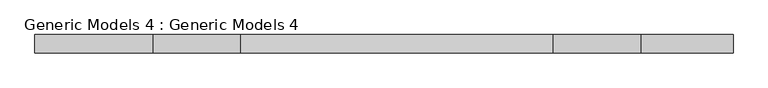
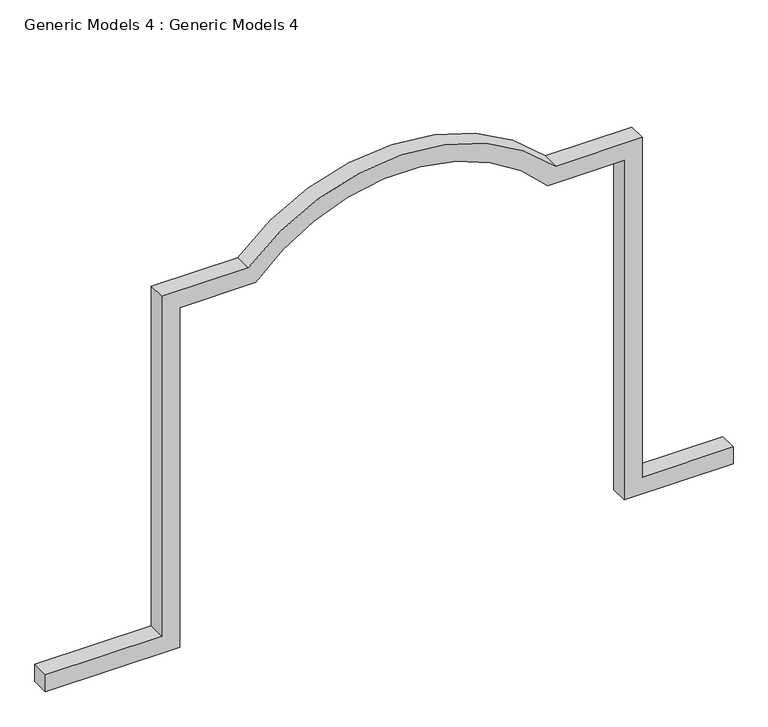
"""IFC4 building model written with IfcOpenShell, lengths in millimetres: proxy geometry, Generic Models 4 : Generic Models 4."""

from ifc_helpers import new_model, si_unit, point, frame, frame_2d, origin, place, context, project, spatial, polyline, circle_curve, trimmed, segment, composite_curve, outline, extrude, source, transform, mapped, element, save


def generic_models_4_generic_models_4_3df0761b(model_context):
    return source(origin(), model_context, "Body", "SweptSolid", [
        extrude(outline(composite_curve([segment(polyline([(2343.9330823, -11036.1236584), (2343.9330823, -10604.3236584)]), True, "CONTINUOUS"), segment(trimmed(circle_curve(frame_2d((1611.4465902, -9778.8236584)), 1103.6243524), [point((2343.9330823, -10604.3236584))], [point((2343.9330823, -8953.3236584))], True, "CARTESIAN"), True, "CONTINUOUS"), segment(polyline([(2343.9330823, -8953.3236584), (2343.9330823, -8521.5236584), (312.5949901, -8521.5236584), (312.5949901, -7905.5736584), (414.1949901, -7905.5736584), (414.1949901, -8419.9236584), (2445.5330823, -8419.9236584), (2445.5330823, -8908.8435074)]), True, "CONTINUOUS"), segment(trimmed(circle_curve(frame_2d((1611.4465902, -9778.8236584)), 1205.2243524), [point((2445.5330823, -8908.8435074))], [point((2445.5330823, -10648.8038094))], False, "CARTESIAN"), True, "CONTINUOUS"), segment(polyline([(2445.5330823, -10648.8038094), (2445.5330823, -11137.7236584), (414.1949901, -11137.7236584), (414.1949901, -11796.2293601), (312.5949901, -11796.2293601), (312.5949901, -11036.1236584), (2343.9330823, -11036.1236584)]), True, "CONTINUOUS")], self_intersect=False)), frame((0.0, -13741.802305, 0.0), z_axis=(0.0, 1.0, 0.0), x_axis=(0.0, 0.0, 1.0)), (0.0, 0.0, 1.0), 101.6),
    ])


if __name__ == "__main__":
    model = new_model("IFC4")
    model_context = context("Model", 3, world=origin())
    ifc_project = project(units=[si_unit("LENGTHUNIT", "METRE", prefix="MILLI")], contexts=[model_context])
    site = spatial("IfcSite", under=ifc_project)
    building = spatial("IfcBuilding", under=site)
    placement = place(None, origin())
    generic_models_4_generic_models_4_shape = generic_models_4_generic_models_4_3df0761b(model_context)
    element("IfcBuildingElementProxy", 1, Name="Generic Models 4 : Generic Models 4", ObjectType="Generic Models 4 : Generic Models 4", at=placement, inside=building, context=model_context, shape_type="MappedRepresentation", body=[
        mapped(generic_models_4_generic_models_4_shape, transform((0.0, 0.0, 0.0), x_axis=(1.0, 0.0, 0.0), y_axis=(0.0, 1.0, 0.0), z_axis=(0.0, 0.0, 1.0))),
    ])
    save(model, "model.ifc")

# Revit data of these elements
# Element 1 (IfcBuildingElementProxy, "Generic Models 4 : Generic Models 4")
#   Materials on its faces: "white colour"
# Materials
#   "white colour": class "Generic", colour RGB 120 120 120, transparency 0, Cost = 0
